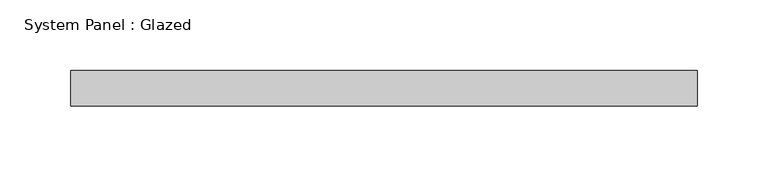
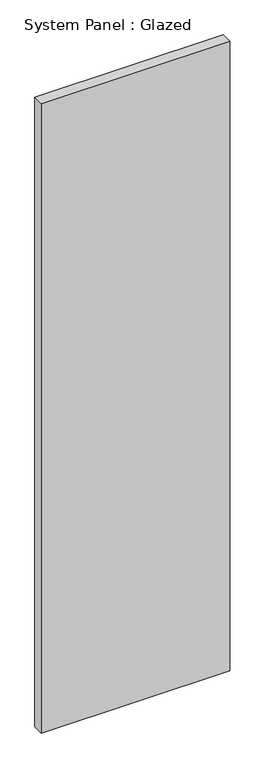
"""IFC4 building model written with IfcOpenShell, lengths in millimetres: plate geometry, System Panel : Glazed."""

from ifc_helpers import new_model, si_unit, origin, origin_with_axes, place, context, project, spatial, polyline, outline, extrude, source, transform, mapped, element, save


def system_panel_glazed_e232d9b5(model_context):
    return source(origin(), model_context, "Body", "SweptSolid", [
        extrude(outline(polyline([(222.25, 19.05), (-222.25, 19.05), (-222.25, 44.45), (222.25, 44.45), (222.25, 19.05)])), origin_with_axes(), (0.0, 0.0, 1.0), 1569.2528693),
    ])


if __name__ == "__main__":
    model = new_model("IFC4")
    model_context = context("Model", 3, world=origin())
    ifc_project = project(units=[si_unit("LENGTHUNIT", "METRE", prefix="MILLI")], contexts=[model_context])
    site = spatial("IfcSite", under=ifc_project)
    building = spatial("IfcBuilding", under=site)
    placement = place(None, origin())
    system_panel_glazed_shape = system_panel_glazed_e232d9b5(model_context)
    element("IfcPlate", 1, ObjectType="System Panel : Glazed", at=placement, inside=building, context=model_context, shape_type="MappedRepresentation", body=[
        mapped(system_panel_glazed_shape, transform((0.0, 0.0, 0.0), x_axis=(1.0, 0.0, 0.0), y_axis=(0.0, 1.0, 0.0), z_axis=(0.0, 0.0, 1.0))),
    ])
    save(model, "model.ifc")

# Revit data of these elements
# Type "System Panel : Glazed"
#   Construction Type Id = "GSP4R"
#   Analytic Construction = "1/8 in Pilkington single glazing"
#   Visual Light Transmittance = 0.9
#   Solar Heat Gain Coefficient = 0.86
#   Heat Transfer Coefficient (U) = 1.18115 BTU/(h·ft²·°F)
#   Define Thermal Properties by = 1
# Element 1 (IfcPlate, "System Panel : Glazed")
#   Materials on its faces: "Glass"
# Materials
#   "Glass": class "Glass", colour RGB 0 128 192, transparency 0.75, Description = "Soda Lime Glass", Cost = 0
